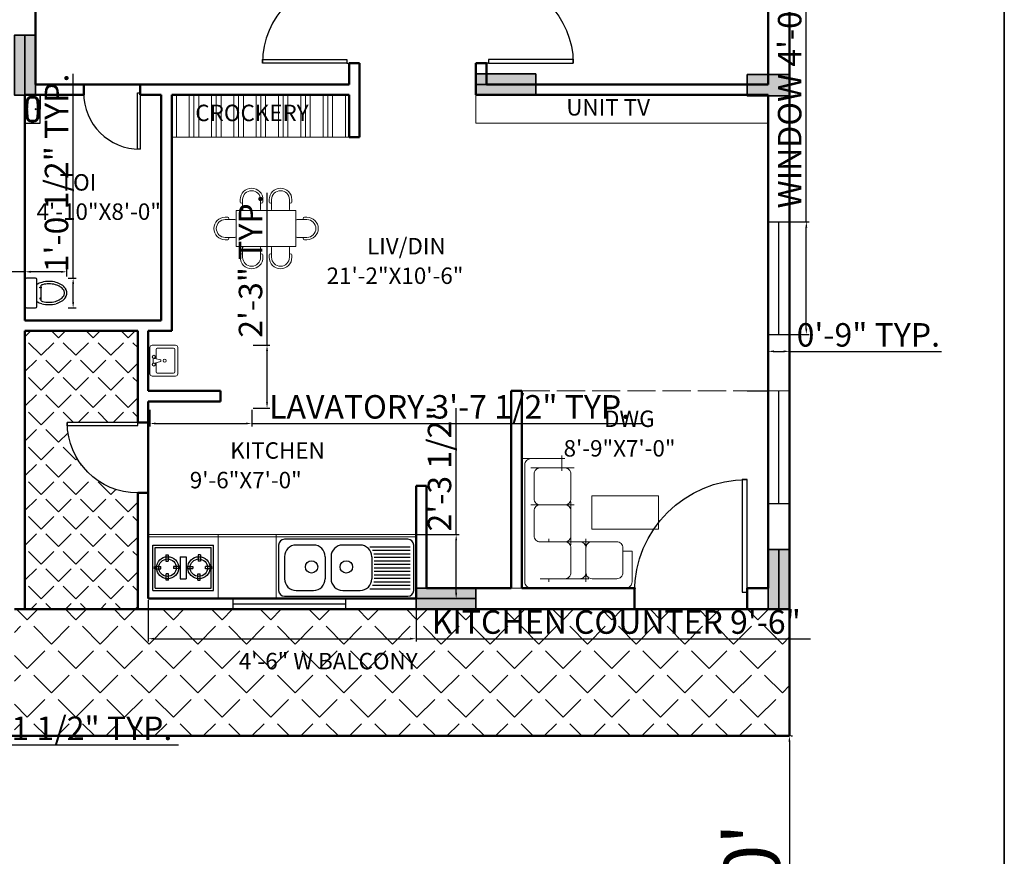
# Model space of a CAD drawing. Units: inches. Extents: x 2214 to 3937, y 762 to 2085.
# Tile 8 of 9: x 3243 to 3663, y 1424 to 1780. Entities that reach past the tile are written whole.
import ezdxf

# ---------------------------------------------------------------- set-up
doc = ezdxf.new("R2010")
doc.units = ezdxf.units.IN
doc.linetypes.add('ACAD_ISO02W100', pattern=[15, 12, -3])
for name, color, linetype, lineweight in [('A-ANNO-TEXT', 7, 'Continuous', 18), ('A-AREA-IDEN', 7, 'Continuous', 25), ('A-CASE', 252, 'Continuous', 18), ('A-CASE-PATT', 252, 'Continuous', 13), ('A-COLS', 5, 'Continuous', 35), ('A-FLOR-FIXT', 9, 'Continuous', 18), ('A-FLOR-PATT', 116, 'Continuous', 13), ('A-FURN', 8, 'Continuous', 18), ('A-WALL-OVHD', 20, 'ACAD_ISO02W100', 18), ('C-ANNO-DIMS', 2, 'Continuous', 18), ('C-PROP', 3, 'Continuous', 35), ('door', 122, 'Continuous', 25), ('wall', 20, 'Continuous', 50), ('window', 4, 'Continuous', 25)]:
    doc.layers.add(name, color=color, linetype=linetype, lineweight=lineweight)
doc.layers.add('NOI THAT', color=42, linetype='Continuous')
doc.layers.add('THIET-BI', color=21, linetype='Continuous')
doc.styles.add('ATT', font='romans.shx')
doc.styles.get("Standard").update_dxf_attribs({"font": 'arial.ttf'})
doc.dimstyles.new('ISO-25', dxfattribs={"dimtxt": 10, "dimasz": 2.5, "dimexe": 1.25, "dimexo": 0.625, "dimtad": 1, "dimdec": 1, "dimlunit": 4, "dimtxsty": 'Standard', "dimcen": 2.5, "dimadec": 0, "dimazin": 0, "dimtfac": 1, "dimtdec": 1, "dimtmove": 0, "dimatfit": 3, "dimfxl": 1, "dimarcsym": 0})

# ---------------------------------------------------------------- blocks, each defined once
blk = doc.blocks.new('*U2')
for p, q in [((0, 0), (0, -6)), ((40, 0), (40, -6))]:
    blk.add_line(p, q)
blk.add_lwpolyline([(0, 0), (0, 40), (1.75, 40), (1.75, 0)], close=True)
blk.add_arc((0, 0), 40, 0, 90)
blk = doc.blocks.new('A$C5AA626B0')
for p, q in [((661, 1672), (661, 1732)), ((721, 1488), (721, 1732)), ((1171, 1732), (1171, 1488)), ((1231, 1732), (1231, 1672)), ((1386, 1732), (1386, 1672)), ((1446, 1732), (1446, 1488)), ((1896, 1488), (1896, 1732)), ((1956, 1672), (1956, 1732)), ((285, 1293), (345, 1293)), ((558, 1458), (2058, 1458)), ((558, 558), (558, 1458)), ((1476, 1458), (1866, 1458)), ((2058, 1458), (2058, 558)), ((2272, 1293), (2332, 1293)), ((285, 1233), (528, 1233)), ((558, 1203), (558, 813)), ((2058, 813), (2058, 1203)), ((2088, 1233), (2332, 1233)), ((528, 783), (285, 783)), ((2332, 783), (2088, 783)), ((345, 723), (285, 723)), ((2058, 558), (558, 558)), ((721, 528), (721, 285)), ((1171, 285), (1171, 528)), ((1446, 285), (1446, 528)), ((1476, 558), (1866, 558)), ((1896, 528), (1896, 285)), ((2332, 723), (2272, 723)), ((661, 345), (661, 285)), ((1231, 285), (1231, 345)), ((1386, 285), (1386, 345)), ((1956, 345), (1956, 285))]:
    blk.add_line(p, q)
for centre, radius, start, end in [((946, 1732), 285, 0, 180), ((1671, 1732), 285, 0, 180), ((946, 1732), 225, 0, 180), ((1671, 1732), 225, 0, 180), ((691, 1672), 30, 180, 0), ((751, 1488), 30, 180, 270), ((1141, 1488), 30, 270, 0), ((1201, 1672), 30, 180, 0), ((1416, 1672), 30, 180, 0), ((1476, 1488), 30, 180, 270), ((1866, 1488), 30, 270, 0), ((1926, 1672), 30, 180, 0), ((285, 1008), 285, 90, 270), ((345, 1263), 30, 270, 90), ((2272, 1263), 30, 90, 270), ((2332, 1008), 285, 270, 90), ((285, 1008), 225, 90, 270), ((528, 1203), 30, 0, 90), ((2088, 1203), 30, 90, 180), ((2332, 1008), 225, 270, 90), ((345, 753), 30, 270, 90), ((528, 813), 30, 270, 0), ((2088, 813), 30, 180, 270), ((2272, 753), 30, 90, 270), ((751, 528), 30, 90, 180), ((1141, 528), 30, 0, 90), ((1476, 528), 30, 90, 180), ((1866, 528), 30, 0, 90), ((691, 345), 30, 0, 180), ((946, 285), 285, 180, 0), ((946, 285), 225, 180, 0), ((1201, 345), 30, 0, 180), ((1416, 345), 30, 0, 180), ((1671, 285), 285, 180, 0), ((1671, 285), 225, 180, 0), ((1926, 345), 30, 0, 180)]:
    blk.add_arc(centre, radius, start, end)
blk = doc.blocks.new('A$C1D6C0704')
for p, q in [((0, 550), (2300, 550)), ((0, 0), (0, 550)), ((0, 530), (2300, 530)), ((600, 0), (600, 550)), ((1100, 0), (1100, 550)), ((2300, 550), (2300, 0)), ((2300, 0), (0, 0))]:
    blk.add_line(p, q)
at = {"layer": 'NOI THAT'}
for p, q in [((2230, 510), (1170, 510)), ((40, 70), (40, 460)), ((40, 460), (560, 460)), ((60, 90), (60, 440)), ((60, 440), (540, 440)), ((540, 90), (540, 440)), ((560, 70), (560, 460)), ((1120, 460), (1120, 70)), ((1420, 460), (1270, 460)), ((1820, 460), (1670, 460)), ((1904.7, 445), (2250, 445)), ((2280, 70), (2280, 460)), ((151.4, 375), (151.4, 320)), ((151.4, 375), (171.4, 375)), ((171.4, 375), (171.4, 320)), ((275, 360), (325, 360)), ((275, 360), (275, 170)), ((325, 360), (325, 170)), ((448.6, 375), (428.6, 375)), ((428.6, 375), (428.6, 320)), ((448.6, 375), (448.6, 320)), ((1170, 360), (1170, 170)), ((1520, 360), (1520, 170)), ((1570, 360), (1570, 170)), ((1920, 360), (1920, 170)), ((1926.7, 415), (2250, 415)), ((1937.4, 385), (2250, 385)), ((1940, 355), (2250, 355)), ((53.4, 255), (53.4, 275)), ((53.4, 275), (108.4, 275)), ((53.4, 255), (108.4, 255)), ((108.4, 255), (108.4, 275)), ((151.4, 320), (171.4, 320)), ((271.4, 277), (216.4, 277)), ((216.4, 277), (216.4, 257)), ((271.4, 257), (216.4, 257)), ((271.4, 277), (271.4, 257)), ((328.6, 277), (383.6, 277)), ((328.6, 277), (328.6, 257)), ((328.6, 257), (383.6, 257)), ((383.6, 277), (383.6, 257)), ((448.6, 320), (428.6, 320)), ((491.6, 255), (491.6, 275)), ((546.6, 275), (491.6, 275)), ((546.6, 255), (491.6, 255)), ((546.6, 255), (546.6, 275)), ((1940, 325), (2250, 325)), ((1940, 295), (2250, 295)), ((1940, 265), (2250, 265)), ((153.4, 157), (153.4, 212)), ((173.4, 212), (153.4, 212)), ((173.4, 157), (173.4, 212)), ((275, 170), (325, 170)), ((426.6, 157), (426.6, 212)), ((426.6, 212), (446.6, 212)), ((446.6, 157), (446.6, 212)), ((1940, 235), (2250, 235)), ((1940, 205), (2250, 205)), ((1940, 175), (2250, 175)), ((60, 90), (540, 90)), ((173.4, 157), (153.4, 157)), ((426.6, 157), (446.6, 157)), ((1904.7, 85), (2250, 85)), ((1926.7, 115), (2250, 115)), ((1937.4, 145), (2250, 145)), ((40, 70), (560, 70)), ((1170, 20), (2230, 20)), ((1270, 70), (1420, 70)), ((1670, 70), (1820, 70))]:
    blk.add_line(p, q, dxfattribs=at)
for centre, radius in [((165.5, 265.1), 95), ((165.5, 265.1), 75), ((434.5, 265.1), 95), ((434.5, 265.1), 75), ((1402.9, 271.7), 53.2), ((1701.1, 271.7), 53.2)]:
    blk.add_circle(centre, radius, dxfattribs=at)
for centre, radius, start, end in [((1170, 460), 50, 90, 180), ((2230, 460), 50, 0, 90), ((1270, 360), 100, 90, 180), ((1420, 360), 100, 0, 90), ((1670, 360), 100, 90, 180), ((1820, 360), 100, 0, 90), ((1270, 170), 100, 180, 270), ((1420, 170), 100, 270, 0), ((1670, 170), 100, 180, 270), ((1820, 170), 100, 270, 0), ((1170, 70), 50, 180, 270), ((2230, 70), 50, 270, 0)]:
    blk.add_arc(centre, radius, start, end, dxfattribs=at)
blk = doc.blocks.new('15PLAV06')
at = {"color": 0, "linetype": 'ByBlock'}
for p, q in [((0, 8.5), (0, -8.5)), ((16.5, 10), (1.5, 10)), ((4, 1.25), (4, 7.25)), ((4.75, 8), (15.25, 8)), ((16, 7.25), (16, -7.25)), ((18, -8.5), (18, 8.5)), ((2, -1.5), (2, 1.5)), ((7, 0.5), (3, 1.5)), ((7, -0.5), (7, 0.5)), ((3, -1.5), (7, -0.5)), ((4, -7.25), (4, -1.25)), ((1.5, -10), (16.5, -10)), ((15.25, -8), (4.75, -8))]:
    blk.add_line(p, q, dxfattribs=at)
for centre in [(2.5, 2.5), (9.5, 0), (2.5, -2.5)]:
    blk.add_circle(centre, 1, dxfattribs=at)
for centre, radius, start, end in [((1.5, 8.5), 1.5, 90, 180), ((4.75, 7.25), 0.75, 90, 180), ((15.25, 7.25), 0.75, 0, 90), ((16.5, 8.5), 1.5, 0, 90), ((1.5, -8.5), 1.5, 180, 270), ((4.75, -7.25), 0.75, 180, 270), ((15.25, -7.25), 0.75, 270, 0), ((16.5, -8.5), 1.5, 270, 0)]:
    blk.add_arc(centre, radius, start, end, dxfattribs=at)
at = {"color": 0, "linetype": 'ByBlock', "style": 'ATT'}
for tag, p, flags in [('ITEM', (0, -20), 3), ('ROOM_NUMBER', (0, -29), 1)]:
    blk.add_attdef(tag, p, '', height=6, dxfattribs=dict(at, flags=flags))
blk = doc.blocks.new('A$C65B13726')
at = {"layer": 'THIET-BI'}
for p, q in [((0, 400), (0, 200)), ((0, 400), (375, 400)), ((134, 362), (621, 360)), ((375, 291), (357, 291)), ((357, 291), (393, 291)), ((375, 291), (375, 309)), ((375, 309), (375, 274)), ((134, 39), (616, 39))]:
    blk.add_line(p, q, dxfattribs=at)
blk.add_lwpolyline([(0, 400), (0, 0), (750, 0), (750, 400)], close=True, dxfattribs=at)
blk.add_lwpolyline([(714, 200), (714, 240, 0.341607), (621, 360), (598, 366, 0.001439), (593, 367, 0.035276), (375, 382, 0.035276), (157, 367, 0.001439), (152, 366), (129, 360, 0.341607), (36, 240), (36, 200), (36, 161, 0.341607), (129, 40), (152, 34, 0.001439), (157, 33, 0.035276), (375, 18, 0.035276), (593, 33, 0.001439), (598, 34), (621, 40, 0.341607), (714, 161)], format="xyb", close=True, dxfattribs=at)
for points in [[(323, 348, 0.026733), (162, 334, 0.000876), (159, 333), (137, 327, 0.341782), (70, 240), (70, 161, 0.341782), (137, 73), (159, 67, 0.000876), (162, 67, 0.026747), (323, 52, 0.035276)], [(337, 337, 0.028876), (163, 323, 0.00069), (161, 322), (140, 317, 0.341861), (81, 240), (81, 160, 0.341861), (140, 83), (161, 78, 0.00069), (163, 77, 0.028898), (337, 63, 0.035276)], [(407, 348, 0.00526), (375, 349, 0.005313), (343, 348, 0.000876)], [(394, 338, 0.003179), (375, 338, 0.003179), (356, 338, 0.00069)], [(375, 382), (375, 382, 0.025118)], [(375, 382), (375, 382, 0.035276)], [(669, 200), (669, 240, 0.341861), (610, 317), (589, 322, 0.00069), (587, 323, 0.028876), (413, 337, 0.003179)], [(680, 200), (680, 240, 0.341782), (613, 327), (591, 333, 0.000876), (588, 334, 0.026733), (427, 348, 0.006503)], [(343, 52, 0.005316), (375, 52, 0.005263), (407, 52, 0.000876)], [(356, 62, 0.003135), (375, 62, 0.003135), (394, 62, 0.00069)], [(375, 17), (375, 17, 0.035276)], [(413, 63, 0.028961), (587, 77, 0.00069), (589, 78), (610, 83, 0.341861), (669, 160), (669, 200)], [(427, 52, 0.026747), (588, 67, 0.000876), (591, 67), (613, 73, 0.341782), (680, 161), (680, 200)]]:
    blk.add_lwpolyline(points, format="xyb", dxfattribs=at)
blk.add_circle((375, 291), 14.5, dxfattribs=at)
for centre, radius, start, end in [((375, 400), 73.6, 211.9576, 327.7237), ((324, 352), 19.1, 310.8832, 28.9258), ((375, 400), 65.2, 239.0852, 300.5961), ((426, 351), 19.1, 150.7555, 228.798), ((375, 0), 73.6, 32.2763, 148.0424), ((324, 48), 19.1, 331.0742, 49.1168), ((375, 0), 65.2, 59.4039, 120.9148), ((426, 49), 19.1, 131.202, 209.2445)]:
    blk.add_arc(centre, radius, start, end, dxfattribs=at)
blk = doc.blocks.new('A$C5AF77858')
at = {"layer": 'THIET-BI'}
for p, q in [((0, 675), (0, 525)), ((475, 700), (25, 700)), ((500, 525), (500, 675)), ((25, 500), (475, 500)), ((117, 430), (383, 430)), ((154, 452), (154, 430)), ((164, 452), (154, 452)), ((154, 430), (164, 430)), ((164, 430), (164, 452)), ((336, 430), (336, 452)), ((336, 452), (346, 452)), ((346, 430), (336, 430)), ((346, 452), (346, 430))]:
    blk.add_line(p, q, dxfattribs=at)
for centre, radius, start, end in [((25, 675), 25, 90, 180), ((475, 675), 25, 0, 90), ((25, 525), 25, 180, 270), ((384, 334), 323, 149.0966, 164.9269), ((116, 334), 323, 15.0731, 30.9034), ((475, 525), 25, 270, 0), ((514, 299), 458, 164.9269, 180), ((514, 299), 418, 164.9269, 180), ((384, 334), 283, 160.176, 164.9269), ((116, 334), 283, 15.0731, 19.824), ((-14, 299), 418, 0, 15.0731), ((-14, 299), 458, 0, 15.0731), ((514, 299), 458, 180, 195.0731), ((384, 264), 323, 195.0731, 213.0315), ((514, 299), 418, 180, 195.0731), ((384, 264), 283, 195.0731, 213.0315), ((116, 264), 283, 326.9685, 344.9269), ((116, 264), 323, 326.9685, 344.9269), ((-14, 299), 418, 344.9269, 0), ((-14, 299), 458, 344.9269, 0), ((302, 210), 226, 213.0315, 237.5002), ((302, 210), 186, 213.0315, 237.5002), ((250, 129), 129, 237.5002, 270), ((250, 129), 89.3, 237.5002, 270), ((250, 129), 89.3, 270, 302.4998), ((250, 129), 129, 270, 302.4998), ((198, 210), 186, 302.4998, 326.9685), ((198, 210), 226, 302.4998, 326.9685)]:
    blk.add_arc(centre, radius, start, end, dxfattribs=at)
blk = doc.blocks.new('*D23')
at = {"layer": 'C-ANNO-DIMS', "color": 0, "lineweight": -2, "ltscale": 0.3, "transparency": 16777216}
for p, q in [((3571.06, 1472.72), (3571.06, 1357.72)), ((3571.68, 1475.22), (3572.31, 1475.22)), ((3571.68, 1355.22), (3572.31, 1355.22))]:
    blk.add_line(p, q, dxfattribs=at)
at = {"layer": 'C-ANNO-DIMS', "color": 0, "ltscale": 0.3, "transparency": 16777216}
for points in [[(3570.64, 1472.72), (3571.47, 1472.72), (3571.06, 1475.22)], [(3570.64, 1357.72), (3571.47, 1357.72), (3571.06, 1355.22)]]:
    blk.add_solid(points, dxfattribs=at)
at = {"layer": 'Defpoints', "color": 0, "ltscale": 0.3, "transparency": 16777216}
for p in [(3571.06, 1475.22), (3571.06, 1355.22), (3571.06, 1355.22)]:
    blk.add_point(p, dxfattribs=at)
at = {"layer": 'C-ANNO-DIMS', "color": 0, "ltscale": 0.3, "transparency": 16777216, "insert": (3558.18, 1415.22), "char_height": 24, "attachment_point": 5, "rotation": 90}
blk.add_mtext("10'", dxfattribs=at)
blk = doc.blocks.new('COL-25_5X9')
at = {"ltscale": 0.3}
h = blk.add_hatch(color=256, dxfattribs=at)
h.dxf.hatch_style = 1
h.paths.add_polyline_path([(25.5, 0), (25.5, 9), (0, 9), (0, 0)])
for p, q in [((25.5, 9), (25.5, 0)), ((0, 4.5), (25.5, 4.5)), ((0, 4.5), (0, 0)), ((0, 0), (4.5, 0))]:
    blk.add_line(p, q)
blk.add_lwpolyline([(0, 9), (25.5, 9), (25.5, 0), (0, 0)], close=True, dxfattribs=at)
blk = doc.blocks.new('COL-18X9')
at = {"ltscale": 0.3}
h = blk.add_hatch(color=256, dxfattribs=at)
h.dxf.hatch_style = 1
h.paths.add_polyline_path([(18, 0), (18, 9), (0, 9), (0, 0)])
blk.add_lwpolyline([(0, 9), (18, 9), (18, 0), (0, 0)], close=True, dxfattribs=at)
blk = doc.blocks.new('WIN-48X9')
for p, q in [((0, 48), (9, 48)), ((0, 0), (9, 0))]:
    blk.add_line(p, q)
at = {"ltscale": 0.3}
blk.add_line((4.5, 0), (4.5, 48), dxfattribs=at)
blk = doc.blocks.new('*D33')
at = {"layer": 'C-ANNO-DIMS', "color": 0, "lineweight": -2, "ltscale": 0.3, "transparency": 16777216}
for p, q in [((3133.06, 1474.59), (3133.06, 1470.14)), ((3158.56, 1474.59), (3158.56, 1470.14)), ((3135.56, 1471.39), (3156.06, 1471.39)), ((3158.56, 1471.39), (3310.87, 1471.39))]:
    blk.add_line(p, q, dxfattribs=at)
at = {"layer": 'C-ANNO-DIMS', "color": 0, "ltscale": 0.3, "transparency": 16777216}
for points in [[(3135.56, 1471.81), (3135.56, 1470.98), (3133.06, 1471.39)], [(3156.06, 1471.81), (3156.06, 1470.98), (3158.56, 1471.39)]]:
    blk.add_solid(points, dxfattribs=at)
at = {"layer": 'Defpoints', "color": 0, "ltscale": 0.3, "transparency": 16777216}
for p in [(3133.06, 1475.22), (3158.56, 1475.22), (3158.56, 1471.39)]:
    blk.add_point(p, dxfattribs=at)
at = {"layer": 'C-ANNO-DIMS', "color": 0, "ltscale": 0.3, "transparency": 16777216, "insert": (3235.96, 1477.19), "char_height": 10, "attachment_point": 5}
blk.add_mtext('COLUMN 2\'-1 1/2" TYP.', dxfattribs=at)
blk = doc.blocks.new('*D41')
at = {"layer": 'C-ANNO-DIMS', "color": 0, "lineweight": -2, "ltscale": 0.3, "transparency": 16777216}
for p, q in [((3578.26, 1694.22), (3578.26, 1824.51)), ((3571.68, 1694.22), (3579.51, 1694.22)), ((3578.26, 1648.72), (3578.26, 1691.72)), ((3571.68, 1646.22), (3579.51, 1646.22))]:
    blk.add_line(p, q, dxfattribs=at)
at = {"layer": 'C-ANNO-DIMS', "color": 0, "ltscale": 0.3, "transparency": 16777216}
for points in [[(3577.84, 1691.72), (3578.67, 1691.72), (3578.26, 1694.22)], [(3577.84, 1648.72), (3578.67, 1648.72), (3578.26, 1646.22)]]:
    blk.add_solid(points, dxfattribs=at)
at = {"layer": 'Defpoints', "color": 0, "ltscale": 0.3, "transparency": 16777216}
for p in [(3571.06, 1694.22), (3578.26, 1694.22), (3571.06, 1646.22)]:
    blk.add_point(p, dxfattribs=at)
at = {"layer": 'C-ANNO-DIMS', "color": 0, "ltscale": 0.3, "transparency": 16777216, "insert": (3572.46, 1760.61), "char_height": 10, "attachment_point": 5, "rotation": 90}
blk.add_mtext('WINDOW 4\'-0" TYP.', dxfattribs=at)
blk = doc.blocks.new('*D42')
at = {"layer": 'C-ANNO-DIMS', "color": 0, "lineweight": -2, "ltscale": 0.3, "transparency": 16777216}
for p, q in [((3562.06, 1645.59), (3562.06, 1637.77)), ((3571.06, 1645.59), (3571.06, 1637.77)), ((3564.56, 1639.02), (3568.56, 1639.02)), ((3571.06, 1639.02), (3635.76, 1639.02))]:
    blk.add_line(p, q, dxfattribs=at)
at = {"layer": 'C-ANNO-DIMS', "color": 0, "ltscale": 0.3, "transparency": 16777216}
for points in [[(3564.56, 1639.44), (3564.56, 1638.6), (3562.06, 1639.02)], [(3568.56, 1639.44), (3568.56, 1638.6), (3571.06, 1639.02)]]:
    blk.add_solid(points, dxfattribs=at)
at = {"layer": 'Defpoints', "color": 0, "ltscale": 0.3, "transparency": 16777216}
for p in [(3562.06, 1646.22), (3571.06, 1646.22), (3571.06, 1639.02)]:
    blk.add_point(p, dxfattribs=at)
at = {"layer": 'C-ANNO-DIMS', "color": 0, "ltscale": 0.3, "transparency": 16777216, "insert": (3604.66, 1644.75), "char_height": 10, "attachment_point": 5}
blk.add_mtext('0\'-9" TYP.', dxfattribs=at)
blk = doc.blocks.new('*D49')
at = {"layer": 'C-ANNO-DIMS', "color": 0, "lineweight": -2, "ltscale": 0.3, "transparency": 16777216}
for p, q in [((3245.56, 1672.91), (3153.29, 1672.91)), ((3245.56, 1670.86), (3245.56, 1674.16)), ((3260.89, 1672.91), (3248.06, 1672.91)), ((3263.39, 1670.86), (3263.39, 1674.16))]:
    blk.add_line(p, q, dxfattribs=at)
at = {"layer": 'C-ANNO-DIMS', "color": 0, "ltscale": 0.3, "transparency": 16777216}
for points in [[(3248.06, 1673.33), (3248.06, 1672.5), (3245.56, 1672.91)], [(3260.89, 1673.33), (3260.89, 1672.5), (3263.39, 1672.91)]]:
    blk.add_solid(points, dxfattribs=at)
at = {"layer": 'Defpoints', "color": 0, "ltscale": 0.3, "transparency": 16777216}
for p in [(3245.56, 1672.91), (3245.56, 1670.24), (3263.39, 1670.24)]:
    blk.add_point(p, dxfattribs=at)
at = {"layer": 'C-ANNO-DIMS', "color": 0, "ltscale": 0.3, "transparency": 16777216, "insert": (3198.17, 1678.71), "char_height": 10, "attachment_point": 5}
blk.add_mtext('WC 1\'-6" TYP.', dxfattribs=at)
blk = doc.blocks.new('*D50')
at = {"layer": 'C-ANNO-DIMS', "color": 0, "lineweight": -2, "ltscale": 0.3, "transparency": 16777216}
for p, q in [((3266.06, 1670.24), (3266.06, 1757.3)), ((3264.01, 1670.24), (3267.31, 1670.24)), ((3266.06, 1660), (3266.06, 1667.74)), ((3264.01, 1657.5), (3267.31, 1657.5))]:
    blk.add_line(p, q, dxfattribs=at)
at = {"layer": 'C-ANNO-DIMS', "color": 0, "ltscale": 0.3, "transparency": 16777216}
for points in [[(3265.65, 1667.74), (3266.48, 1667.74), (3266.06, 1670.24)], [(3265.65, 1660), (3266.48, 1660), (3266.06, 1657.5)]]:
    blk.add_solid(points, dxfattribs=at)
at = {"layer": 'Defpoints', "color": 0, "ltscale": 0.3, "transparency": 16777216}
for p in [(3263.39, 1670.24), (3266.06, 1670.24), (3263.39, 1657.5)]:
    blk.add_point(p, dxfattribs=at)
at = {"layer": 'C-ANNO-DIMS', "color": 0, "ltscale": 0.3, "transparency": 16777216, "insert": (3260.27, 1715.02), "char_height": 10, "attachment_point": 5, "rotation": 90}
blk.add_mtext('1\'-0 1/2" TYP.', dxfattribs=at)
blk = doc.blocks.new('*D53')
at = {"layer": 'C-ANNO-DIMS', "color": 0, "lineweight": -2, "ltscale": 0.3, "transparency": 16777216}
for p, q in [((3298.06, 1533.09), (3298.06, 1515.37)), ((3412.06, 1533.09), (3412.06, 1515.37)), ((3300.56, 1516.62), (3409.56, 1516.62)), ((3412.06, 1516.62), (3580.1, 1516.62))]:
    blk.add_line(p, q, dxfattribs=at)
at = {"layer": 'C-ANNO-DIMS', "color": 0, "ltscale": 0.3, "transparency": 16777216}
for points in [[(3300.56, 1517.04), (3300.56, 1516.2), (3298.06, 1516.62)], [(3409.56, 1517.04), (3409.56, 1516.2), (3412.06, 1516.62)]]:
    blk.add_solid(points, dxfattribs=at)
at = {"layer": 'Defpoints', "color": 0, "ltscale": 0.3, "transparency": 16777216}
for p in [(3298.06, 1533.72), (3412.06, 1533.72), (3412.06, 1516.62)]:
    blk.add_point(p, dxfattribs=at)
at = {"layer": 'C-ANNO-DIMS', "color": 0, "ltscale": 0.3, "transparency": 16777216, "insert": (3497.33, 1522.42), "char_height": 10, "attachment_point": 5}
blk.add_mtext('KITCHEN COUNTER 9\'-6"', dxfattribs=at)
blk = doc.blocks.new('*D54')
at = {"layer": 'C-ANNO-DIMS', "color": 0, "lineweight": -2, "ltscale": 0.3, "transparency": 16777216}
for p, q in [((3429.16, 1560.98), (3429.16, 1614.78)), ((3412.68, 1560.98), (3430.41, 1560.98)), ((3429.16, 1536.22), (3429.16, 1558.48)), ((3412.68, 1533.72), (3430.41, 1533.72))]:
    blk.add_line(p, q, dxfattribs=at)
at = {"layer": 'C-ANNO-DIMS', "color": 0, "ltscale": 0.3, "transparency": 16777216}
for points in [[(3428.74, 1558.48), (3429.57, 1558.48), (3429.16, 1560.98)], [(3428.74, 1536.22), (3429.57, 1536.22), (3429.16, 1533.72)]]:
    blk.add_solid(points, dxfattribs=at)
at = {"layer": 'Defpoints', "color": 0, "ltscale": 0.3, "transparency": 16777216}
for p in [(3412.06, 1560.98), (3429.16, 1560.98), (3412.06, 1533.72)]:
    blk.add_point(p, dxfattribs=at)
at = {"layer": 'C-ANNO-DIMS', "color": 0, "ltscale": 0.3, "transparency": 16777216, "insert": (3423.36, 1589.13), "char_height": 10, "attachment_point": 5, "rotation": 90}
blk.add_mtext('2\'-3 1/2"', dxfattribs=at)
blk = doc.blocks.new('*D59')
at = {"layer": 'C-ANNO-DIMS', "color": 0, "lineweight": -2, "ltscale": 0.3, "transparency": 16777216}
for p, q in [((3298.76, 1614.17), (3298.76, 1607.04)), ((3342.12, 1614.17), (3342.12, 1607.04)), ((3301.26, 1608.29), (3339.62, 1608.29)), ((3342.12, 1608.29), (3508.09, 1608.29))]:
    blk.add_line(p, q, dxfattribs=at)
at = {"layer": 'C-ANNO-DIMS', "color": 0, "ltscale": 0.3, "transparency": 16777216}
for points in [[(3301.26, 1608.71), (3301.26, 1607.87), (3298.76, 1608.29)], [(3339.62, 1608.71), (3339.62, 1607.87), (3342.12, 1608.29)]]:
    blk.add_solid(points, dxfattribs=at)
at = {"layer": 'Defpoints', "color": 0, "ltscale": 0.3, "transparency": 16777216}
for p in [(3298.76, 1614.79), (3342.12, 1614.79), (3342.12, 1608.29)]:
    blk.add_point(p, dxfattribs=at)
at = {"layer": 'C-ANNO-DIMS', "color": 0, "ltscale": 0.3, "transparency": 16777216, "insert": (3426.36, 1614.09), "char_height": 10, "attachment_point": 5}
blk.add_mtext('LAVATORY 3\'-7 1/2" TYP.', dxfattribs=at)
blk = doc.blocks.new('*D60')
at = {"layer": 'C-ANNO-DIMS', "color": 0, "lineweight": -2, "ltscale": 0.3, "transparency": 16777216}
for p, q in [((3348.62, 1641.64), (3348.62, 1706.52)), ((3342.74, 1641.64), (3349.87, 1641.64)), ((3348.62, 1617.29), (3348.62, 1639.14)), ((3342.74, 1614.79), (3349.87, 1614.79))]:
    blk.add_line(p, q, dxfattribs=at)
at = {"layer": 'C-ANNO-DIMS', "color": 0, "ltscale": 0.3, "transparency": 16777216}
for points in [[(3348.21, 1639.14), (3349.04, 1639.14), (3348.62, 1641.64)], [(3348.21, 1617.29), (3349.04, 1617.29), (3348.62, 1614.79)]]:
    blk.add_solid(points, dxfattribs=at)
at = {"layer": 'Defpoints', "color": 0, "ltscale": 0.3, "transparency": 16777216}
for p in [(3342.12, 1641.64), (3348.62, 1641.64), (3342.12, 1614.79)]:
    blk.add_point(p, dxfattribs=at)
at = {"layer": 'C-ANNO-DIMS', "color": 0, "ltscale": 0.3, "transparency": 16777216, "insert": (3342.89, 1675.33), "char_height": 10, "attachment_point": 5, "rotation": 90}
blk.add_mtext('2\'-3" TYP.', dxfattribs=at)

msp = doc.modelspace()

# ---------------------------------------------------------------- hatches: boundary and pattern name
at = {"layer": 'A-CASE-PATT'}
h = msp.add_hatch(dxfattribs=at)
h.set_pattern_fill('GOST_GROUND', color=256, scale=0.95, angle=45)
h.paths.add_polyline_path([(3383.56, 1748.22), (3308.06, 1748.22), (3308.06, 1730.22), (3383.56, 1730.22)])
at = {"layer": 'A-FLOR-PATT', "ltscale": 0.3}
h = msp.add_hatch(dxfattribs=at)
h.set_pattern_fill('ANGLE', color=256, scale=1.5, angle=45)
h.set_pattern_definition([(45, (0, 0), (-7.40871, 7.40871), [7.62, -2.8575]), (135, (0, 0), (-7.40871, -7.40871), [7.62, -2.8575])])
h.paths.add_polyline_path([(3293.56, 1578.72, -0.401453), (3263.59, 1607.41), (3263.56, 1607.41), (3263.56, 1608.72), (3293.56, 1608.72), (3293.56, 1647.72), (3245.56, 1647.72), (3245.56, 1529.22), (3293.56, 1529.22)])
h = msp.add_hatch(dxfattribs=at)
h.set_pattern_fill('ANGLE', color=256, scale=2.1, angle=45)
h.set_pattern_definition([(45, (0, 0), (-10.372196, 10.372196), [10.668, -4.0005]), (135, (0, 0), (-10.372196, -10.372196), [10.668, -4.0005])])
h.paths.add_polyline_path([(3571.06, 1529.18), (3562.06, 1529.18), (3241.06, 1529.22), (3241.06, 1475.22), (3571.06, 1475.22)])

# ---------------------------------------------------------------- linework, layer by layer
at = {"layer": 'A-CASE'}
for p, q in [((3437.56, 1748.22), (3437.56, 1736.22)), ((3437.56, 1736.22), (3562.06, 1736.22)), ((3383.56, 1730.22), (3308.06, 1730.22))]:
    msp.add_line(p, q, dxfattribs=at)
at = {"layer": 'A-FURN'}
for points in [[(3475.42, 1593.32), (3457.06, 1593.32)], [(3474.11, 1588.07), (3474.11, 1594.63)], [(3474.11, 1593.32), (3474.11, 1589.38)], [(3460.99, 1589.38), (3479.36, 1589.38)], [(3460.99, 1589.38), (3479.36, 1589.38)], [(3460.99, 1573.64), (3479.36, 1573.64)], [(3460.99, 1573.64), (3479.36, 1573.64)], [(3478.05, 1574.95), (3478.05, 1556.59)], [(3464.93, 1557.9), (3479.36, 1557.9)], [(3464.93, 1557.9), (3479.36, 1557.9)], [(3464.93, 1557.9), (3466.03, 1557.9)], [(3464.93, 1557.9), (3469.97, 1557.9)], [(3467.34, 1557.9), (3485.71, 1557.9)], [(3468.66, 1559.21), (3468.66, 1557.9)], [(3468.66, 1557.9), (3468.66, 1559.21)], [(3468.66, 1557.9), (3468.66, 1559.21)], [(3483.09, 1557.9), (3497.52, 1557.9)], [(3484.4, 1540.84), (3484.4, 1559.21)], [(3504.08, 1553.96), (3500.14, 1553.96)], [(3466.03, 1542.15), (3479.36, 1542.15)], [(3466.03, 1542.15), (3469.97, 1542.15)], [(3467.34, 1542.15), (3485.71, 1542.15)], [(3468.66, 1540.84), (3468.66, 1542.15)], [(3468.66, 1540.84), (3468.66, 1542.15)], [(3468.66, 1542.15), (3468.66, 1540.84)], [(3447.94, 1538.22), (3474.17, 1538.22)], [(3475.42, 1538.22), (3457.06, 1538.22)], [(3488.81, 1538.22), (3505.66, 1538.22)]]:
    msp.add_lwpolyline(points, dxfattribs=at)
for points in [[(3474.11, 1593.32), (3460.99, 1593.32, 0.414214), (3458.37, 1590.69), (3458.37, 1540.84, 0.414214), (3460.99, 1538.22), (3474.11, 1538.22, 0.506261)], [(3464.93, 1557.9), (3475.42, 1557.9, -0.414214), (3478.05, 1555.27), (3478.05, 1544.78, -0.414214), (3475.42, 1542.15), (3464.93, 1542.15)], [(3471.28, 1557.9), (3481.77, 1557.9, -0.414214), (3484.4, 1555.27), (3484.4, 1544.78, -0.414214), (3481.77, 1542.15), (3471.28, 1542.15)], [(3467.34, 1538.22), (3501.45, 1538.22, 0.414214), (3504.08, 1540.84), (3504.08, 1553.96)], [(3468.66, 1544.78, -0.000004), (3468.66, 1544.78)]]:
    msp.add_lwpolyline(points, format="xyb", dxfattribs=at)
for points in [[(3464.93, 1589.38), (3475.42, 1589.38, -0.414214), (3478.05, 1586.76), (3478.05, 1576.26, -0.414214), (3475.42, 1573.64), (3464.93, 1573.64, -0.414214), (3462.31, 1576.26), (3462.31, 1586.76, -0.414214)], [(3464.93, 1573.64), (3475.42, 1573.64, -0.414214), (3478.05, 1571.02), (3478.05, 1560.52, -0.414214), (3475.42, 1557.9), (3464.93, 1557.9, -0.414214), (3462.31, 1560.52), (3462.31, 1571.02, -0.414214)], [(3484.4, 1544.78), (3484.4, 1555.27, -0.414214), (3487.02, 1557.9), (3497.52, 1557.9, -0.414214), (3500.14, 1555.27), (3500.14, 1544.78, -0.414214), (3497.52, 1542.15), (3487.02, 1542.15, -0.414214)]]:
    msp.add_lwpolyline(points, format="xyb", close=True, dxfattribs=at)
msp.add_lwpolyline([(3515.29, 1577.41), (3515.29, 1563.29), (3486.87, 1563.29), (3486.87, 1577.41)], close=True, dxfattribs=at)
at = {"layer": 'A-WALL-OVHD'}
msp.add_line((3457.06, 1622.22), (3571.06, 1622.22), dxfattribs=at)
at = {"layer": 'C-PROP'}
msp.add_line((3662.56, 2003.22), (3662.56, 1355.22), dxfattribs=at)
at = {"layer": 'wall'}
for p, q in [((3571.06, 1911.72), (3571.06, 1475.22)), ((3250.06, 1752.72), (3250.06, 1902.72)), ((3562.06, 1902.72), (3562.06, 1752.72)), ((3383.56, 1752.72), (3383.56, 1761.72)), ((3383.56, 1761.72), (3388.06, 1761.72)), ((3388.06, 1730.22), (3388.06, 1761.72)), ((3437.56, 1748.22), (3437.56, 1761.72)), ((3442.06, 1761.72), (3437.56, 1761.72)), ((3442.06, 1752.72), (3442.06, 1761.72)), ((3250.06, 1752.72), (3383.56, 1752.72)), ((3270.56, 1748.22), (3270.56, 1752.72)), ((3294.56, 1748.22), (3294.56, 1752.72)), ((3442.06, 1752.72), (3562.06, 1752.72)), ((3245.56, 1748.22), (3270.56, 1748.22)), ((3245.56, 1652.22), (3245.56, 1748.22)), ((3294.56, 1748.22), (3303.56, 1748.22)), ((3303.56, 1652.22), (3303.56, 1748.22)), ((3308.06, 1647.72), (3308.06, 1748.22)), ((3308.06, 1748.22), (3383.56, 1748.22)), ((3383.56, 1730.22), (3383.56, 1748.22)), ((3437.56, 1748.22), (3562.06, 1748.22)), ((3562.06, 1748.22), (3562.06, 1538.22)), ((3383.56, 1730.22), (3388.06, 1730.22)), ((3245.56, 1652.22), (3303.56, 1652.22)), ((3245.56, 1529.22), (3245.56, 1647.72)), ((3245.56, 1647.72), (3293.56, 1647.72)), ((3293.56, 1608.72), (3293.56, 1647.72)), ((3298.06, 1647.72), (3308.06, 1647.72)), ((3298.06, 1622.22), (3298.06, 1647.72)), ((3328.86, 1622.22), (3298.06, 1622.22)), ((3328.86, 1622.22), (3328.86, 1617.72)), ((3457.06, 1622.22), (3452.56, 1622.22)), ((3452.56, 1538.22), (3452.56, 1622.22)), ((3457.06, 1538.22), (3457.06, 1622.22)), ((3298.06, 1533.72), (3298.06, 1617.72)), ((3328.86, 1617.72), (3298.06, 1617.72)), ((3298.06, 1608.72), (3293.56, 1608.72)), ((3412.06, 1533.72), (3412.06, 1581.72)), ((3416.56, 1581.72), (3412.06, 1581.72)), ((3416.56, 1538.22), (3416.56, 1581.72)), ((3293.56, 1529.22), (3293.56, 1578.72)), ((3298.06, 1578.72), (3293.56, 1578.72)), ((3452.56, 1538.22), (3416.56, 1538.22)), ((3505.06, 1538.22), (3457.06, 1538.22)), ((3505.06, 1538.22), (3505.06, 1529.22)), ((3562.06, 1538.22), (3553.06, 1538.22)), ((3553.06, 1538.22), (3553.06, 1529.22)), ((3412.06, 1533.72), (3298.06, 1533.72)), ((3571.06, 1529.22), (3241.06, 1529.22)), ((3571.06, 1475.22), (2674.06, 1475.22))]:
    msp.add_line(p, q, dxfattribs=at)
at = {"layer": 'window'}
for p, q in [((3553.06, 1622.22), (3562.06, 1622.22)), ((3562.06, 1574.22), (3571.06, 1574.22))]:
    msp.add_line(p, q, dxfattribs=at)
at = {"layer": 'window', "ltscale": 0.3}
for p, q in [((3566.56, 1574.22), (3566.56, 1622.22)), ((3334.06, 1533.72), (3334.06, 1529.22)), ((3334.06, 1531.47), (3382.06, 1531.47)), ((3382.06, 1533.72), (3382.06, 1529.22))]:
    msp.add_line(p, q, dxfattribs=at)

# ---------------------------------------------------------------- block references
at = {"layer": 'A-COLS'}
for p, rotation in [((3241.06, 1773.68), 270.0000000000005), ((3562.06, 1554.68), 270.0000000000027)]:
    msp.add_blockref('COL-25_5X9', p, dxfattribs=dict(at, rotation=rotation))
for name, p in [('COL-25_5X9', (3437.56, 1748.22)), ('COL-18X9', (3553.06, 1747.91)), ('COL-25_5X9', (3412.06, 1529.22))]:
    msp.add_blockref(name, p, dxfattribs=at)
at = {"layer": 'A-FLOR-FIXT'}
for name, p, xscale, yscale, zscale, rotation in [('A$C65B13726', (3245.56, 1748.18), 0.0160009442456078, 0.0160009442456078, 0.0160009442456078, 270), ('A$C5AF77858', (3263.39, 1657.5), 0.0254713121376822, 0.0254713121376822, 0.0254713121376822, 90)]:
    msp.add_blockref(name, p, dxfattribs=dict(at, xscale=xscale, yscale=yscale, zscale=zscale, rotation=rotation))
for name, p, xscale, yscale, zscale in [('15PLAV06', (3298.76, 1635.05), 0.6595085966356266, 0.6595085966356266, 0.6595085966356266), ('A$C1D6C0704', (3298.06, 1533.72), 0.0495652178024062, 0.0495652178024062, 0.0495652178024062)]:
    msp.add_blockref(name, p, dxfattribs=dict(at, xscale=xscale, yscale=yscale, zscale=zscale))
at = {"layer": 'A-FURN', "xscale": 0.0169743344463681, "yscale": 0.0169743344463681, "zscale": 0.0169743344463681}
msp.add_blockref('A$C5AA626B0', (3326.01, 1674.24), dxfattribs=at)
at = {"layer": 'door'}
for p, xscale, yscale, zscale, rotation in [((3382.66, 1761.72), 0.9, 0.9, 0.9, 90), ((3442.96, 1761.72), -0.9, 0.9, 0.9, 270), ((3294.56, 1749.12), 0.6000000000000069, 0.6000000000000069, 0.6000000000000069, 180), ((3293.56, 1608.72), -0.75, 0.75, 0.75, 90)]:
    msp.add_blockref('*U2', p, dxfattribs=dict(at, xscale=xscale, yscale=yscale, zscale=zscale, rotation=rotation))
at = {"layer": 'door', "xscale": -1.199999999999988, "yscale": 1.199999999999988, "zscale": 1.199999999999988}
msp.add_blockref('*U2', (3553.06, 1536.42), dxfattribs=at)
at = {"layer": 'window'}
msp.add_blockref('WIN-48X9', (3562.06, 1646.22), dxfattribs=at)

# ---------------------------------------------------------------- texts
at = {"layer": 'A-ANNO-TEXT', "ltscale": 0.3}
for s, p in [('CROCKERY', (3318.09, 1737.09)), ('UNIT TV', (3476.04, 1739.47))]:
    msp.add_text(s, height=7, dxfattribs=at).set_placement(p)
at = {"layer": 'A-AREA-IDEN', "ltscale": 0.3}
for s, p in [('TOI', (3260.32, 1707.5)), ('4\'-10"X8\'-0"', (3250.49, 1695.04)), ('LIV/DIN', (3391.2, 1680.34)), ('21\'-2"X10\'-6"', (3373.98, 1667.74)), ('DWG', (3492.12, 1606.81)), ('8\'-9"X7\'-0"', (3474.9, 1594.21)), ('KITCHEN', (3332.95, 1593.29)), ('9\'-6"X7\'-0"', (3315.73, 1580.69)), ('4\'-6" W BALCONY', (3336.59, 1503.58))]:
    msp.add_text(s, height=7, dxfattribs=at).set_placement(p)

# ---------------------------------------------------------------- dimensions: what is measured, and where the dimension line sits
at = {"layer": 'C-ANNO-DIMS', "ltscale": 0.3}
for base, p1, p2, angle, text, picture, middle in [((3578.26, 1694.22), (3571.06, 1646.22), (3571.06, 1694.22), 90, 'WINDOW <> TYP.', '*D41', (3572.46, 1760.61)), ((3266.06, 1670.24), (3263.39, 1657.5), (3263.39, 1670.24), 90, '<> TYP.', '*D50', (3260.27, 1715.02)), ((3348.6219, 1641.6435), (3342.1186, 1614.7935), (3342.1186, 1641.6435), 90, '<> TYP.', '*D60', (3342.8877, 1675.3312)), ((3245.56, 1672.91), (3263.39, 1670.24), (3245.56, 1670.24), 180, 'WC <> TYP.', '*D49', (3198.17, 1678.71))]:
    dim = msp.add_linear_dim(base=base, p1=p1, p2=p2, angle=angle, text=text, dimstyle='ISO-25', override={"dimdec": 1, "dimlfac": 1, "dimrnd": 0, "dimzin": 1, "dimdsep": 46, "dimlunit": 4, "dimfrac": 2}, dxfattribs=at)
    dim.commit()
    dim.dimension.update_dxf_attribs({"geometry": picture, "text_midpoint": middle})
for base, p1, p2, text, picture, middle in [((3571.06, 1639.02), (3562.06, 1646.22), (3571.06, 1646.22), '<> TYP.', '*D42', (3604.66, 1644.75)), ((3342.12, 1608.29), (3298.76, 1614.79), (3342.12, 1614.79), 'LAVATORY <> TYP.', '*D59', (3426.36, 1614.09)), ((3412.06, 1516.62), (3298.06, 1533.72), (3412.06, 1533.72), 'KITCHEN COUNTER <>', '*D53', (3497.33, 1522.42)), ((3158.56, 1471.39), (3133.06, 1475.22), (3158.56, 1475.22), 'COLUMN <> TYP.', '*D33', (3235.96, 1477.19))]:
    dim = msp.add_linear_dim(base=base, p1=p1, p2=p2, text=text, dimstyle='ISO-25', override={"dimdec": 1, "dimlfac": 1, "dimrnd": 0, "dimzin": 1, "dimdsep": 46, "dimlunit": 4, "dimfrac": 2}, dxfattribs=at)
    dim.commit()
    dim.dimension.update_dxf_attribs({"geometry": picture, "text_midpoint": middle})
for base, p1, p2, override, picture, middle in [((3429.16, 1560.98), (3412.06, 1533.72), (3412.06, 1560.98), {"dimdec": 1, "dimlfac": 1, "dimrnd": 0, "dimzin": 1, "dimdsep": 46, "dimlunit": 4, "dimfrac": 2}, '*D54', (3423.36, 1589.13)), ((3571.06, 1355.22), (3571.06, 1475.22), (3571.06, 1355.22), {"dimtxt": 24, "dimclrd": 0, "dimclre": 0, "dimclrt": 0}, '*D23', (3558.18, 1415.22))]:
    dim = msp.add_linear_dim(base=base, p1=p1, p2=p2, angle=90, dimstyle='ISO-25', override=override, dxfattribs=at)
    dim.commit()
    dim.dimension.update_dxf_attribs({"geometry": picture, "text_midpoint": middle})

doc.saveas('drawing.dxf')
